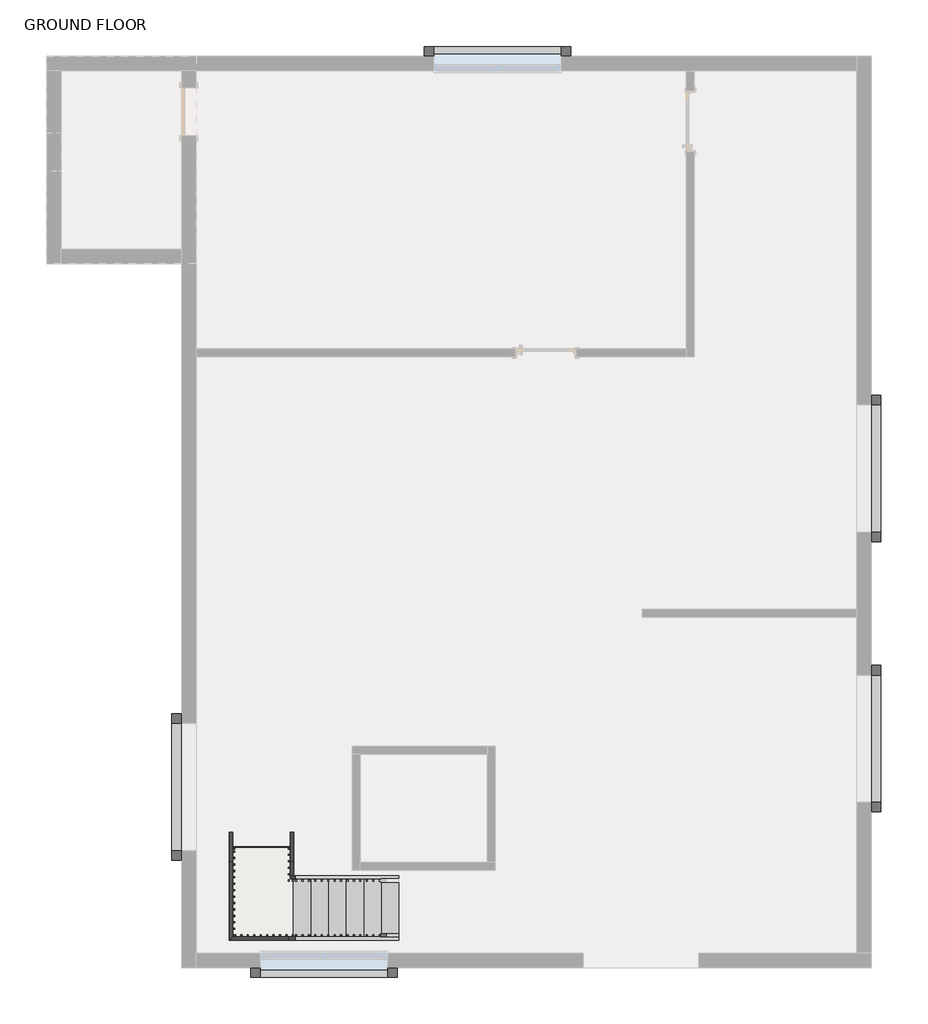
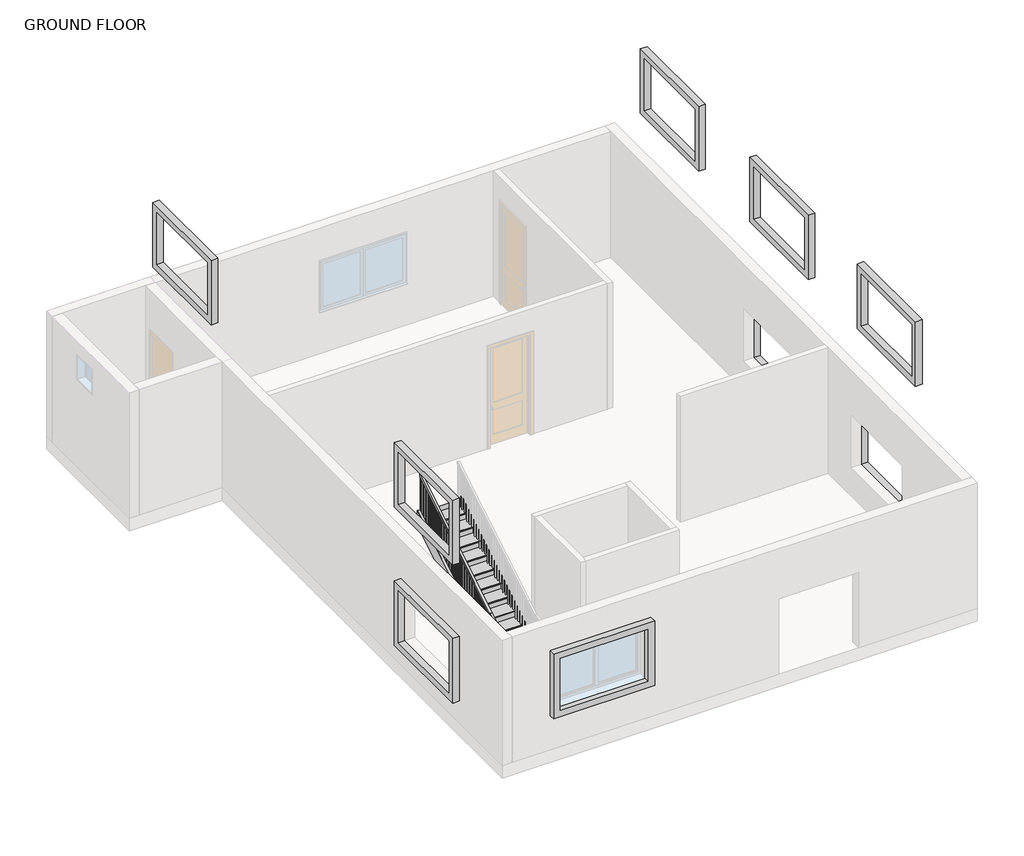
# One storey, part 2 of 2: 7 members, 4 proxies, 2 stair flights, 1 railing, 1 slab.
"""IFC4 building model written with IfcOpenShell, lengths in millimetres."""

from ifc_helpers import new_model, si_unit, frame, origin, place, context, project, spatial, polyline, outline, extrude, faceted_brep, transform, mapped, element, save
from components import generic_models_3_generic_models_3_62885dc4, generic_models_4_generic_models_4_3a3d2180, generic_models_7_generic_models_7_0c2edacf, generic_models_8_generic_models_8_56cf2c1e, non_monolithic_landing_e724ba9d, stair_flight_0804820e, stair_flight_c801c68a

model = new_model("IFC4")

# Units and contexts
model_context = context("Model", 3, world=origin())
ifc_project = project(units=[si_unit("LENGTHUNIT", "METRE", prefix="MILLI")], contexts=[model_context])

# Site, building, storey
site = spatial("IfcSite", under=ifc_project)
building = spatial("IfcBuilding", under=site)
storey = spatial("IfcBuildingStorey", under=building, Name="GROUND FLOOR", Elevation=304.8)

# Proxies
placement = place(None, origin())
generic_models_3_generic_models_3_shape = generic_models_3_generic_models_3_62885dc4(model_context)
element("IfcBuildingElementProxy", 1, Name="Generic Models 3 : Generic Models 3", ObjectType="Generic Models 3 : Generic Models 3", at=placement, inside=storey, context=model_context, shape_type="MappedRepresentation", body=[
    mapped(generic_models_3_generic_models_3_shape, transform((0.0, 0.0, 0.0), x_axis=(1.0, 0.0, 0.0), y_axis=(0.0, 1.0, 0.0), z_axis=(0.0, 0.0, 1.0))),
])
generic_models_4_generic_models_4_shape = generic_models_4_generic_models_4_3a3d2180(model_context)
element("IfcBuildingElementProxy", 2, Name="Generic Models 4 : Generic Models 4", ObjectType="Generic Models 4 : Generic Models 4", at=placement, inside=storey, context=model_context, shape_type="MappedRepresentation", body=[
    mapped(generic_models_4_generic_models_4_shape, transform((0.0, 0.0, 0.0), x_axis=(1.0, 0.0, 0.0), y_axis=(0.0, 1.0, 0.0), z_axis=(0.0, 0.0, 1.0))),
])
generic_models_7_generic_models_7_shape = generic_models_7_generic_models_7_0c2edacf(model_context)
element("IfcBuildingElementProxy", 3, Name="Generic Models 7 : Generic Models 7", ObjectType="Generic Models 7 : Generic Models 7", at=placement, inside=storey, context=model_context, shape_type="MappedRepresentation", body=[
    mapped(generic_models_7_generic_models_7_shape, transform((0.0, 0.0, 0.0), x_axis=(1.0, 0.0, 0.0), y_axis=(0.0, 1.0, 0.0), z_axis=(0.0, 0.0, 1.0))),
])
generic_models_8_generic_models_8_shape = generic_models_8_generic_models_8_56cf2c1e(model_context)
element("IfcBuildingElementProxy", 4, Name="Generic Models 8 : Generic Models 8", ObjectType="Generic Models 8 : Generic Models 8", at=placement, inside=storey, context=model_context, shape_type="MappedRepresentation", body=[
    mapped(generic_models_8_generic_models_8_shape, transform((0.0, 0.0, 0.0), x_axis=(1.0, 0.0, 0.0), y_axis=(0.0, 1.0, 0.0), z_axis=(0.0, 0.0, 1.0))),
])

# Members
element("IfcMember", 5, ObjectType="Stringer - 2\" Width", at=placement, inside=storey, context=model_context, shape_type="SweptSolid", body=[
    extrude(outline(polyline([(304.8, -3322.4601025), (516.914512, -3322.4601025), (1566.3333333, -5054.0011578), (1261.5333333, -5139.1556143), (304.8, -3560.5456143), (304.8, -3322.4601025)])), frame((0.0, -3834.257314, 0.0), z_axis=(0.0, 1.0, 0.0), x_axis=(0.0, 0.0, 1.0)), (0.0, 0.0, 1.0), 50.8),
])
element("IfcMember", 6, ObjectType="Stringer - 2\" Width", at=placement, inside=storey, context=model_context, shape_type="SweptSolid", body=[
    extrude(outline(polyline([(304.8, -3322.4601025), (516.914512, -3322.4601025), (1556.1357187, -5037.1750936), (1199.7269571, -5037.1750936), (304.8, -3560.5456143), (304.8, -3322.4601025)])), frame((0.0, -2869.057314, 0.0), z_axis=(0.0, 1.0, 0.0), x_axis=(0.0, 0.0, 1.0)), (0.0, 0.0, 1.0), 50.8),
])
element("IfcMember", 7, ObjectType="Stringer - 2\" Width", at=placement, inside=storey, context=model_context, shape_type="SweptSolid", body=[
    extrude(outline(polyline([(-2530.2317367, 1261.5333333), (-2615.3861932, 1566.3333333), (402.8727516, 3395.5811786), (402.8727516, 3039.1724171), (-2530.2317367, 1261.5333333)])), frame((-6002.3750936, 0.0, 0.0), z_axis=(1.0, 0.0, 0.0), x_axis=(0.0, 1.0, 0.0)), (0.0, 0.0, 1.0), 50.8),
])
element("IfcMember", 8, ObjectType="Stringer - 2\" Width", at=placement, inside=storey, context=model_context, shape_type="SweptSolid", body=[
    extrude(outline(polyline([(-2530.2317367, 1261.5333333), (-2615.3861932, 1566.3333333), (402.8727516, 3395.5811786), (402.8727516, 3039.1724171), (-2530.2317367, 1261.5333333)])), frame((-5037.1750936, 0.0, 0.0), z_axis=(1.0, 0.0, 0.0), x_axis=(0.0, 1.0, 0.0)), (0.0, 0.0, 1.0), 50.8),
])
element("IfcMember", 9, ObjectType="Stringer - 2\" Width", at=placement, inside=storey, context=model_context, shape_type="Brep", body=[
    faceted_brep([(-5951.5750936, -2615.3861932, 1566.3333333), (-6002.3750936, -2615.3861932, 1566.3333333), (-6002.3750936, -3834.257314, 1566.3333333), (-5951.5750936, -3783.457314, 1566.3333333), (-5951.5750936, -2530.2317367, 1261.5333333), (-5951.5750936, -3783.457314, 1261.5333333), (-6002.3750936, -2530.2317367, 1261.5333333), (-6002.3750936, -3834.257314, 1261.5333333)], [[[0, 1, 2, 3]], [[4, 0, 3, 5]], [[6, 4, 5, 7]], [[1, 6, 7, 2]], [[1, 0, 4, 6]], [[2, 7, 5, 3]]]),
])
element("IfcMember", 10, ObjectType="Stringer - 2\" Width", at=placement, inside=storey, context=model_context, shape_type="Brep", body=[
    faceted_brep([(-5951.5750936, -3783.457314, 1566.3333333), (-6002.3750936, -3834.257314, 1566.3333333), (-5054.0011578, -3834.257314, 1566.3333333), (-5054.0011578, -3783.457314, 1566.3333333), (-5951.5750936, -3783.457314, 1261.5333333), (-5139.1556143, -3783.457314, 1261.5333333), (-6002.3750936, -3834.257314, 1261.5333333), (-5139.1556143, -3834.257314, 1261.5333333)], [[[0, 1, 2, 3]], [[4, 0, 3, 5]], [[6, 4, 5, 7]], [[1, 6, 7, 2]], [[1, 0, 4, 6]], [[2, 7, 5, 3]]]),
])
element("IfcMember", 11, ObjectType="Stringer - 2\" Width", at=placement, inside=storey, context=model_context, shape_type="SweptSolid", body=[
    extrude(outline(polyline([(-2818.257314, 1261.5333333), (-2818.257314, 1566.3333333), (-2615.3861932, 1566.3333333), (-2530.2317367, 1261.5333333), (-2818.257314, 1261.5333333)])), frame((-5037.1750936, 0.0, 0.0), z_axis=(1.0, 0.0, 0.0), x_axis=(0.0, 1.0, 0.0)), (0.0, 0.0, 1.0), 50.8),
])

# Railing
element("IfcRailing", 12, ObjectType="Handrail - Rectangular", at=placement, inside=storey, context=model_context, shape_type="SolidModel", body=[
    faceted_brep([(-3322.4601025, -3783.457314, 1388.5333333), (-3322.4601025, -3783.457314, 1329.1318731), (-3322.4601025, -3732.657314, 1329.1318731), (-3322.4601025, -3732.657314, 1388.5333333), (-4998.8601025, -3783.457314, 2404.5333333), (-5013.0525119, -3783.457314, 2353.7333333), (-5013.0525119, -3732.657314, 2353.7333333), (-4998.8601025, -3732.657314, 2404.5333333), (-5951.5750936, -3783.457314, 2404.5333333), (-5951.5750936, -3783.457314, 2353.7333333), (-5900.7750936, -3732.657314, 2353.7333333), (-5900.7750936, -3732.657314, 2404.5333333), (-5951.5750936, -2670.5272484, 2404.5333333), (-5951.5750936, -2656.334839, 2353.7333333), (-5900.7750936, -2656.334839, 2353.7333333), (-5900.7750936, -2670.5272484, 2404.5333333), (-5951.5750936, -2391.1272484, 2573.8666667), (-5951.5750936, -2364.7975213, 2530.4226168), (-5900.7750936, -2364.7975213, 2530.4226168), (-5900.7750936, -2391.1272484, 2573.8666667), (-5951.5750936, 402.8727516, 4267.2), (-5900.7750936, 402.8727516, 4267.2), (-5900.7750936, 402.8727516, 4207.7985397), (-5951.5750936, 402.8727516, 4207.7985397)], [[[0, 1, 2, 3]], [[1, 0, 4, 5]], [[2, 1, 5, 6]], [[3, 2, 6, 7]], [[0, 3, 7, 4]], [[5, 4, 8, 9]], [[6, 5, 9, 10]], [[7, 6, 10, 11]], [[4, 7, 11, 8]], [[9, 8, 12, 13]], [[10, 9, 13, 14]], [[11, 10, 14, 15]], [[8, 11, 15, 12]], [[13, 12, 16, 17]], [[14, 13, 17, 18]], [[15, 14, 18, 19]], [[12, 15, 19, 16]], [[20, 21, 22, 23]], [[17, 16, 20, 23]], [[18, 17, 23, 22]], [[19, 18, 22, 21]], [[16, 19, 21, 20]]]),
    extrude(outline(polyline([(361.5977516, 4182.7833882), (361.5977516, 3183.4666667), (342.5477516, 3183.4666667), (342.5477516, 4171.2379337), (361.5977516, 4182.7833882)])), frame((-5935.7000936, 0.0, 0.0), z_axis=(1.0, 0.0, 0.0), x_axis=(0.0, 1.0, 0.0)), (0.0, 0.0, 1.0), 19.05),
    extrude(outline(polyline([(259.9977516, 4121.2076307), (259.9977516, 3183.4666667), (240.9477516, 3183.4666667), (240.9477516, 4109.6621761), (259.9977516, 4121.2076307)])), frame((-5935.7000936, 0.0, 0.0), z_axis=(1.0, 0.0, 0.0), x_axis=(0.0, 1.0, 0.0)), (0.0, 0.0, 1.0), 19.05),
    extrude(outline(polyline([(158.3977516, 4059.6318731), (158.3977516, 3183.4666667), (139.3477516, 3183.4666667), (139.3477516, 4048.0864185), (158.3977516, 4059.6318731)])), frame((-5935.7000936, 0.0, 0.0), z_axis=(1.0, 0.0, 0.0), x_axis=(0.0, 1.0, 0.0)), (0.0, 0.0, 1.0), 19.05),
    extrude(outline(polyline([(56.7977516, 3998.0561155), (56.7977516, 3014.1333333), (37.7477516, 3014.1333333), (37.7477516, 3986.510661), (56.7977516, 3998.0561155)])), frame((-5935.7000936, 0.0, 0.0), z_axis=(1.0, 0.0, 0.0), x_axis=(0.0, 1.0, 0.0)), (0.0, 0.0, 1.0), 19.05),
    extrude(outline(polyline([(-44.8022484, 3936.4803579), (-44.8022484, 3014.1333333), (-63.8522484, 3014.1333333), (-63.8522484, 3924.9349034), (-44.8022484, 3936.4803579)])), frame((-5935.7000936, 0.0, 0.0), z_axis=(1.0, 0.0, 0.0), x_axis=(0.0, 1.0, 0.0)), (0.0, 0.0, 1.0), 19.05),
    extrude(outline(polyline([(-146.4022484, 3874.9046004), (-146.4022484, 3014.1333333), (-165.4522484, 3014.1333333), (-165.4522484, 3863.3591458), (-146.4022484, 3874.9046004)])), frame((-5935.7000936, 0.0, 0.0), z_axis=(1.0, 0.0, 0.0), x_axis=(0.0, 1.0, 0.0)), (0.0, 0.0, 1.0), 19.05),
    extrude(outline(polyline([(-248.0022484, 3813.3288428), (-248.0022484, 2844.8), (-267.0522484, 2844.8), (-267.0522484, 3801.7833882), (-248.0022484, 3813.3288428)])), frame((-5935.7000936, 0.0, 0.0), z_axis=(1.0, 0.0, 0.0), x_axis=(0.0, 1.0, 0.0)), (0.0, 0.0, 1.0), 19.05),
    extrude(outline(polyline([(-349.6022484, 3751.7530852), (-349.6022484, 2844.8), (-368.6522484, 2844.8), (-368.6522484, 3740.2076307), (-349.6022484, 3751.7530852)])), frame((-5935.7000936, 0.0, 0.0), z_axis=(1.0, 0.0, 0.0), x_axis=(0.0, 1.0, 0.0)), (0.0, 0.0, 1.0), 19.05),
    extrude(outline(polyline([(-451.2022484, 3690.1773276), (-451.2022484, 2675.4666667), (-470.2522484, 2675.4666667), (-470.2522484, 3678.6318731), (-451.2022484, 3690.1773276)])), frame((-5935.7000936, 0.0, 0.0), z_axis=(1.0, 0.0, 0.0), x_axis=(0.0, 1.0, 0.0)), (0.0, 0.0, 1.0), 19.05),
    extrude(outline(polyline([(-552.8022484, 3628.60157), (-552.8022484, 2675.4666667), (-571.8522484, 2675.4666667), (-571.8522484, 3617.0561155), (-552.8022484, 3628.60157)])), frame((-5935.7000936, 0.0, 0.0), z_axis=(1.0, 0.0, 0.0), x_axis=(0.0, 1.0, 0.0)), (0.0, 0.0, 1.0), 19.05),
    extrude(outline(polyline([(-654.4022484, 3567.0258125), (-654.4022484, 2675.4666667), (-673.4522484, 2675.4666667), (-673.4522484, 3555.4803579), (-654.4022484, 3567.0258125)])), frame((-5935.7000936, 0.0, 0.0), z_axis=(1.0, 0.0, 0.0), x_axis=(0.0, 1.0, 0.0)), (0.0, 0.0, 1.0), 19.05),
    extrude(outline(polyline([(-756.0022484, 3505.4500549), (-756.0022484, 2506.1333333), (-775.0522484, 2506.1333333), (-775.0522484, 3493.9046004), (-756.0022484, 3505.4500549)])), frame((-5935.7000936, 0.0, 0.0), z_axis=(1.0, 0.0, 0.0), x_axis=(0.0, 1.0, 0.0)), (0.0, 0.0, 1.0), 19.05),
    extrude(outline(polyline([(-857.6022484, 3443.8742973), (-857.6022484, 2506.1333333), (-876.6522484, 2506.1333333), (-876.6522484, 3432.3288428), (-857.6022484, 3443.8742973)])), frame((-5935.7000936, 0.0, 0.0), z_axis=(1.0, 0.0, 0.0), x_axis=(0.0, 1.0, 0.0)), (0.0, 0.0, 1.0), 19.05),
    extrude(outline(polyline([(-959.2022484, 3382.2985397), (-959.2022484, 2506.1333333), (-978.2522484, 2506.1333333), (-978.2522484, 3370.7530852), (-959.2022484, 3382.2985397)])), frame((-5935.7000936, 0.0, 0.0), z_axis=(1.0, 0.0, 0.0), x_axis=(0.0, 1.0, 0.0)), (0.0, 0.0, 1.0), 19.05),
    extrude(outline(polyline([(-1060.8022484, 3320.7227822), (-1060.8022484, 2336.8), (-1079.8522484, 2336.8), (-1079.8522484, 3309.1773276), (-1060.8022484, 3320.7227822)])), frame((-5935.7000936, 0.0, 0.0), z_axis=(1.0, 0.0, 0.0), x_axis=(0.0, 1.0, 0.0)), (0.0, 0.0, 1.0), 19.05),
    extrude(outline(polyline([(-1162.4022484, 3259.1470246), (-1162.4022484, 2336.8), (-1181.4522484, 2336.8), (-1181.4522484, 3247.60157), (-1162.4022484, 3259.1470246)])), frame((-5935.7000936, 0.0, 0.0), z_axis=(1.0, 0.0, 0.0), x_axis=(0.0, 1.0, 0.0)), (0.0, 0.0, 1.0), 19.05),
    extrude(outline(polyline([(-1264.0022484, 3197.571267), (-1264.0022484, 2336.8), (-1283.0522484, 2336.8), (-1283.0522484, 3186.0258125), (-1264.0022484, 3197.571267)])), frame((-5935.7000936, 0.0, 0.0), z_axis=(1.0, 0.0, 0.0), x_axis=(0.0, 1.0, 0.0)), (0.0, 0.0, 1.0), 19.05),
    extrude(outline(polyline([(-1365.6022484, 3135.9955094), (-1365.6022484, 2167.4666667), (-1384.6522484, 2167.4666667), (-1384.6522484, 3124.4500549), (-1365.6022484, 3135.9955094)])), frame((-5935.7000936, 0.0, 0.0), z_axis=(1.0, 0.0, 0.0), x_axis=(0.0, 1.0, 0.0)), (0.0, 0.0, 1.0), 19.05),
    extrude(outline(polyline([(-1467.2022484, 3074.4197519), (-1467.2022484, 2167.4666667), (-1486.2522484, 2167.4666667), (-1486.2522484, 3062.8742973), (-1467.2022484, 3074.4197519)])), frame((-5935.7000936, 0.0, 0.0), z_axis=(1.0, 0.0, 0.0), x_axis=(0.0, 1.0, 0.0)), (0.0, 0.0, 1.0), 19.05),
    extrude(outline(polyline([(-1568.8022484, 3012.8439943), (-1568.8022484, 1998.1333333), (-1587.8522484, 1998.1333333), (-1587.8522484, 3001.2985397), (-1568.8022484, 3012.8439943)])), frame((-5935.7000936, 0.0, 0.0), z_axis=(1.0, 0.0, 0.0), x_axis=(0.0, 1.0, 0.0)), (0.0, 0.0, 1.0), 19.05),
    extrude(outline(polyline([(-1670.4022484, 2951.2682367), (-1670.4022484, 1998.1333333), (-1689.4522484, 1998.1333333), (-1689.4522484, 2939.7227822), (-1670.4022484, 2951.2682367)])), frame((-5935.7000936, 0.0, 0.0), z_axis=(1.0, 0.0, 0.0), x_axis=(0.0, 1.0, 0.0)), (0.0, 0.0, 1.0), 19.05),
    extrude(outline(polyline([(-1772.0022484, 2889.6924791), (-1772.0022484, 1998.1333333), (-1791.0522484, 1998.1333333), (-1791.0522484, 2878.1470246), (-1772.0022484, 2889.6924791)])), frame((-5935.7000936, 0.0, 0.0), z_axis=(1.0, 0.0, 0.0), x_axis=(0.0, 1.0, 0.0)), (0.0, 0.0, 1.0), 19.05),
    extrude(outline(polyline([(-1873.6022484, 2828.1167216), (-1873.6022484, 1828.8), (-1892.6522484, 1828.8), (-1892.6522484, 2816.571267), (-1873.6022484, 2828.1167216)])), frame((-5935.7000936, 0.0, 0.0), z_axis=(1.0, 0.0, 0.0), x_axis=(0.0, 1.0, 0.0)), (0.0, 0.0, 1.0), 19.05),
    extrude(outline(polyline([(-1975.2022484, 2766.540964), (-1975.2022484, 1828.8), (-1994.2522484, 1828.8), (-1994.2522484, 2754.9955094), (-1975.2022484, 2766.540964)])), frame((-5935.7000936, 0.0, 0.0), z_axis=(1.0, 0.0, 0.0), x_axis=(0.0, 1.0, 0.0)), (0.0, 0.0, 1.0), 19.05),
    extrude(outline(polyline([(-2076.8022484, 2704.9652064), (-2076.8022484, 1828.8), (-2095.8522484, 1828.8), (-2095.8522484, 2693.4197519), (-2076.8022484, 2704.9652064)])), frame((-5935.7000936, 0.0, 0.0), z_axis=(1.0, 0.0, 0.0), x_axis=(0.0, 1.0, 0.0)), (0.0, 0.0, 1.0), 19.05),
    extrude(outline(polyline([(-2178.4022484, 2643.3894488), (-2178.4022484, 1659.4666667), (-2197.4522484, 1659.4666667), (-2197.4522484, 2631.8439943), (-2178.4022484, 2643.3894488)])), frame((-5935.7000936, 0.0, 0.0), z_axis=(1.0, 0.0, 0.0), x_axis=(0.0, 1.0, 0.0)), (0.0, 0.0, 1.0), 19.05),
    extrude(outline(polyline([(-2280.0022484, 2581.8136913), (-2280.0022484, 1659.4666667), (-2299.0522484, 1659.4666667), (-2299.0522484, 2570.2682367), (-2280.0022484, 2581.8136913)])), frame((-5935.7000936, 0.0, 0.0), z_axis=(1.0, 0.0, 0.0), x_axis=(0.0, 1.0, 0.0)), (0.0, 0.0, 1.0), 19.05),
    extrude(outline(polyline([(-2427.732314, 2492.2803182), (-2427.732314, 1490.1333333), (-2446.782314, 1490.1333333), (-2446.782314, 2480.7348636), (-2427.732314, 2492.2803182)])), frame((-5935.7000936, 0.0, 0.0), z_axis=(1.0, 0.0, 0.0), x_axis=(0.0, 1.0, 0.0)), (0.0, 0.0, 1.0), 19.05),
    extrude(outline(polyline([(-2529.332314, 2430.7045606), (-2529.332314, 1490.1333333), (-2548.382314, 1490.1333333), (-2548.382314, 2419.1591061), (-2529.332314, 2430.7045606)])), frame((-5935.7000936, 0.0, 0.0), z_axis=(1.0, 0.0, 0.0), x_axis=(0.0, 1.0, 0.0)), (0.0, 0.0, 1.0), 19.05),
    extrude(outline(polyline([(-2630.932314, 2369.128803), (-2630.932314, 1490.1333333), (-2649.982314, 1490.1333333), (-2649.982314, 2357.5833485), (-2630.932314, 2369.128803)])), frame((-5935.7000936, 0.0, 0.0), z_axis=(1.0, 0.0, 0.0), x_axis=(0.0, 1.0, 0.0)), (0.0, 0.0, 1.0), 19.05),
    extrude(outline(polyline([(-5935.7000936, -2751.582314), (-5935.7000936, -2732.532314), (-5916.6500936, -2732.532314), (-5916.6500936, -2751.582314), (-5935.7000936, -2751.582314)])), frame((0.0, 0.0, 1490.1333333), z_axis=(0.0, 0.0, 1.0), x_axis=(1.0, 0.0, 0.0)), (0.0, 0.0, 1.0), 863.6),
    extrude(outline(polyline([(-5935.7000936, -2853.182314), (-5935.7000936, -2834.132314), (-5916.6500936, -2834.132314), (-5916.6500936, -2853.182314), (-5935.7000936, -2853.182314)])), frame((0.0, 0.0, 1490.1333333), z_axis=(0.0, 0.0, 1.0), x_axis=(1.0, 0.0, 0.0)), (0.0, 0.0, 1.0), 863.6),
    extrude(outline(polyline([(-5935.7000936, -2954.782314), (-5935.7000936, -2935.732314), (-5916.6500936, -2935.732314), (-5916.6500936, -2954.782314), (-5935.7000936, -2954.782314)])), frame((0.0, 0.0, 1490.1333333), z_axis=(0.0, 0.0, 1.0), x_axis=(1.0, 0.0, 0.0)), (0.0, 0.0, 1.0), 863.6),
    extrude(outline(polyline([(-5935.7000936, -3056.382314), (-5935.7000936, -3037.332314), (-5916.6500936, -3037.332314), (-5916.6500936, -3056.382314), (-5935.7000936, -3056.382314)])), frame((0.0, 0.0, 1490.1333333), z_axis=(0.0, 0.0, 1.0), x_axis=(1.0, 0.0, 0.0)), (0.0, 0.0, 1.0), 863.6),
    extrude(outline(polyline([(-5935.7000936, -3157.982314), (-5935.7000936, -3138.932314), (-5916.6500936, -3138.932314), (-5916.6500936, -3157.982314), (-5935.7000936, -3157.982314)])), frame((0.0, 0.0, 1490.1333333), z_axis=(0.0, 0.0, 1.0), x_axis=(1.0, 0.0, 0.0)), (0.0, 0.0, 1.0), 863.6),
    extrude(outline(polyline([(-5935.7000936, -3259.582314), (-5935.7000936, -3240.532314), (-5916.6500936, -3240.532314), (-5916.6500936, -3259.582314), (-5935.7000936, -3259.582314)])), frame((0.0, 0.0, 1490.1333333), z_axis=(0.0, 0.0, 1.0), x_axis=(1.0, 0.0, 0.0)), (0.0, 0.0, 1.0), 863.6),
    extrude(outline(polyline([(-5935.7000936, -3361.182314), (-5935.7000936, -3342.132314), (-5916.6500936, -3342.132314), (-5916.6500936, -3361.182314), (-5935.7000936, -3361.182314)])), frame((0.0, 0.0, 1490.1333333), z_axis=(0.0, 0.0, 1.0), x_axis=(1.0, 0.0, 0.0)), (0.0, 0.0, 1.0), 863.6),
    extrude(outline(polyline([(-5935.7000936, -3462.782314), (-5935.7000936, -3443.732314), (-5916.6500936, -3443.732314), (-5916.6500936, -3462.782314), (-5935.7000936, -3462.782314)])), frame((0.0, 0.0, 1490.1333333), z_axis=(0.0, 0.0, 1.0), x_axis=(1.0, 0.0, 0.0)), (0.0, 0.0, 1.0), 863.6),
    extrude(outline(polyline([(-5935.7000936, -3564.382314), (-5935.7000936, -3545.332314), (-5916.6500936, -3545.332314), (-5916.6500936, -3564.382314), (-5935.7000936, -3564.382314)])), frame((0.0, 0.0, 1490.1333333), z_axis=(0.0, 0.0, 1.0), x_axis=(1.0, 0.0, 0.0)), (0.0, 0.0, 1.0), 863.6),
    extrude(outline(polyline([(-5935.7000936, -3665.982314), (-5935.7000936, -3646.932314), (-5916.6500936, -3646.932314), (-5916.6500936, -3665.982314), (-5935.7000936, -3665.982314)])), frame((0.0, 0.0, 1490.1333333), z_axis=(0.0, 0.0, 1.0), x_axis=(1.0, 0.0, 0.0)), (0.0, 0.0, 1.0), 863.6),
    extrude(outline(polyline([(-5903.7351025, -3767.582314), (-5922.7851025, -3767.582314), (-5922.7851025, -3748.532314), (-5903.7351025, -3748.532314), (-5903.7351025, -3767.582314)])), frame((0.0, 0.0, 1490.1333333), z_axis=(0.0, 0.0, 1.0), x_axis=(1.0, 0.0, 0.0)), (0.0, 0.0, 1.0), 863.6),
    extrude(outline(polyline([(-5802.1351025, -3767.582314), (-5821.1851025, -3767.582314), (-5821.1851025, -3748.532314), (-5802.1351025, -3748.532314), (-5802.1351025, -3767.582314)])), frame((0.0, 0.0, 1490.1333333), z_axis=(0.0, 0.0, 1.0), x_axis=(1.0, 0.0, 0.0)), (0.0, 0.0, 1.0), 863.6),
    extrude(outline(polyline([(-5700.5351025, -3767.582314), (-5719.5851025, -3767.582314), (-5719.5851025, -3748.532314), (-5700.5351025, -3748.532314), (-5700.5351025, -3767.582314)])), frame((0.0, 0.0, 1490.1333333), z_axis=(0.0, 0.0, 1.0), x_axis=(1.0, 0.0, 0.0)), (0.0, 0.0, 1.0), 863.6),
    extrude(outline(polyline([(-5598.9351025, -3767.582314), (-5617.9851025, -3767.582314), (-5617.9851025, -3748.532314), (-5598.9351025, -3748.532314), (-5598.9351025, -3767.582314)])), frame((0.0, 0.0, 1490.1333333), z_axis=(0.0, 0.0, 1.0), x_axis=(1.0, 0.0, 0.0)), (0.0, 0.0, 1.0), 863.6),
    extrude(outline(polyline([(-5497.3351025, -3767.582314), (-5516.3851025, -3767.582314), (-5516.3851025, -3748.532314), (-5497.3351025, -3748.532314), (-5497.3351025, -3767.582314)])), frame((0.0, 0.0, 1490.1333333), z_axis=(0.0, 0.0, 1.0), x_axis=(1.0, 0.0, 0.0)), (0.0, 0.0, 1.0), 863.6),
    extrude(outline(polyline([(-5395.7351025, -3767.582314), (-5414.7851025, -3767.582314), (-5414.7851025, -3748.532314), (-5395.7351025, -3748.532314), (-5395.7351025, -3767.582314)])), frame((0.0, 0.0, 1490.1333333), z_axis=(0.0, 0.0, 1.0), x_axis=(1.0, 0.0, 0.0)), (0.0, 0.0, 1.0), 863.6),
    extrude(outline(polyline([(-5294.1351025, -3767.582314), (-5313.1851025, -3767.582314), (-5313.1851025, -3748.532314), (-5294.1351025, -3748.532314), (-5294.1351025, -3767.582314)])), frame((0.0, 0.0, 1490.1333333), z_axis=(0.0, 0.0, 1.0), x_axis=(1.0, 0.0, 0.0)), (0.0, 0.0, 1.0), 863.6),
    extrude(outline(polyline([(-5192.5351025, -3767.582314), (-5211.5851025, -3767.582314), (-5211.5851025, -3748.532314), (-5192.5351025, -3748.532314), (-5192.5351025, -3767.582314)])), frame((0.0, 0.0, 1490.1333333), z_axis=(0.0, 0.0, 1.0), x_axis=(1.0, 0.0, 0.0)), (0.0, 0.0, 1.0), 863.6),
    extrude(outline(polyline([(-5090.9351025, -3767.582314), (-5109.9851025, -3767.582314), (-5109.9851025, -3748.532314), (-5090.9351025, -3748.532314), (-5090.9351025, -3767.582314)])), frame((0.0, 0.0, 1490.1333333), z_axis=(0.0, 0.0, 1.0), x_axis=(1.0, 0.0, 0.0)), (0.0, 0.0, 1.0), 863.6),
    extrude(outline(polyline([(2320.1167216, -4957.5851025), (1320.8, -4957.5851025), (1320.8, -4938.5351025), (2308.571267, -4938.5351025), (2320.1167216, -4957.5851025)])), frame((0.0, -3767.582314, 0.0), z_axis=(0.0, 1.0, 0.0), x_axis=(0.0, 0.0, 1.0)), (0.0, 0.0, 1.0), 19.05),
    extrude(outline(polyline([(2258.540964, -4855.9851025), (1320.8, -4855.9851025), (1320.8, -4836.9351025), (2246.9955094, -4836.9351025), (2258.540964, -4855.9851025)])), frame((0.0, -3767.582314, 0.0), z_axis=(0.0, 1.0, 0.0), x_axis=(0.0, 0.0, 1.0)), (0.0, 0.0, 1.0), 19.05),
    extrude(outline(polyline([(2196.9652064, -4754.3851025), (1320.8, -4754.3851025), (1320.8, -4735.3351025), (2185.4197519, -4735.3351025), (2196.9652064, -4754.3851025)])), frame((0.0, -3767.582314, 0.0), z_axis=(0.0, 1.0, 0.0), x_axis=(0.0, 0.0, 1.0)), (0.0, 0.0, 1.0), 19.05),
    extrude(outline(polyline([(2135.3894488, -4652.7851025), (1151.4666667, -4652.7851025), (1151.4666667, -4633.7351025), (2123.8439943, -4633.7351025), (2135.3894488, -4652.7851025)])), frame((0.0, -3767.582314, 0.0), z_axis=(0.0, 1.0, 0.0), x_axis=(0.0, 0.0, 1.0)), (0.0, 0.0, 1.0), 19.05),
    extrude(outline(polyline([(2073.8136913, -4551.1851025), (1151.4666667, -4551.1851025), (1151.4666667, -4532.1351025), (2062.2682367, -4532.1351025), (2073.8136913, -4551.1851025)])), frame((0.0, -3767.582314, 0.0), z_axis=(0.0, 1.0, 0.0), x_axis=(0.0, 0.0, 1.0)), (0.0, 0.0, 1.0), 19.05),
    extrude(outline(polyline([(2012.2379337, -4449.5851025), (1151.4666667, -4449.5851025), (1151.4666667, -4430.5351025), (2000.6924791, -4430.5351025), (2012.2379337, -4449.5851025)])), frame((0.0, -3767.582314, 0.0), z_axis=(0.0, 1.0, 0.0), x_axis=(0.0, 0.0, 1.0)), (0.0, 0.0, 1.0), 19.05),
    extrude(outline(polyline([(1950.6621761, -4347.9851025), (982.1333333, -4347.9851025), (982.1333333, -4328.9351025), (1939.1167216, -4328.9351025), (1950.6621761, -4347.9851025)])), frame((0.0, -3767.582314, 0.0), z_axis=(0.0, 1.0, 0.0), x_axis=(0.0, 0.0, 1.0)), (0.0, 0.0, 1.0), 19.05),
    extrude(outline(polyline([(1889.0864185, -4246.3851025), (982.1333333, -4246.3851025), (982.1333333, -4227.3351025), (1877.540964, -4227.3351025), (1889.0864185, -4246.3851025)])), frame((0.0, -3767.582314, 0.0), z_axis=(0.0, 1.0, 0.0), x_axis=(0.0, 0.0, 1.0)), (0.0, 0.0, 1.0), 19.05),
    extrude(outline(polyline([(1827.510661, -4144.7851025), (812.8, -4144.7851025), (812.8, -4125.7351025), (1815.9652064, -4125.7351025), (1827.510661, -4144.7851025)])), frame((0.0, -3767.582314, 0.0), z_axis=(0.0, 1.0, 0.0), x_axis=(0.0, 0.0, 1.0)), (0.0, 0.0, 1.0), 19.05),
    extrude(outline(polyline([(1765.9349034, -4043.1851025), (812.8, -4043.1851025), (812.8, -4024.1351025), (1754.3894488, -4024.1351025), (1765.9349034, -4043.1851025)])), frame((0.0, -3767.582314, 0.0), z_axis=(0.0, 1.0, 0.0), x_axis=(0.0, 0.0, 1.0)), (0.0, 0.0, 1.0), 19.05),
    extrude(outline(polyline([(1704.3591458, -3941.5851025), (812.8, -3941.5851025), (812.8, -3922.5351025), (1692.8136913, -3922.5351025), (1704.3591458, -3941.5851025)])), frame((0.0, -3767.582314, 0.0), z_axis=(0.0, 1.0, 0.0), x_axis=(0.0, 0.0, 1.0)), (0.0, 0.0, 1.0), 19.05),
    extrude(outline(polyline([(1642.7833882, -3839.9851025), (643.4666667, -3839.9851025), (643.4666667, -3820.9351025), (1631.2379337, -3820.9351025), (1642.7833882, -3839.9851025)])), frame((0.0, -3767.582314, 0.0), z_axis=(0.0, 1.0, 0.0), x_axis=(0.0, 0.0, 1.0)), (0.0, 0.0, 1.0), 19.05),
    extrude(outline(polyline([(1581.2076307, -3738.3851025), (643.4666667, -3738.3851025), (643.4666667, -3719.3351025), (1569.6621761, -3719.3351025), (1581.2076307, -3738.3851025)])), frame((0.0, -3767.582314, 0.0), z_axis=(0.0, 1.0, 0.0), x_axis=(0.0, 0.0, 1.0)), (0.0, 0.0, 1.0), 19.05),
    extrude(outline(polyline([(1519.6318731, -3636.7851025), (643.4666667, -3636.7851025), (643.4666667, -3617.7351025), (1508.0864185, -3617.7351025), (1519.6318731, -3636.7851025)])), frame((0.0, -3767.582314, 0.0), z_axis=(0.0, 1.0, 0.0), x_axis=(0.0, 0.0, 1.0)), (0.0, 0.0, 1.0), 19.05),
    extrude(outline(polyline([(1458.0561155, -3535.1851025), (474.1333333, -3535.1851025), (474.1333333, -3516.1351025), (1446.510661, -3516.1351025), (1458.0561155, -3535.1851025)])), frame((0.0, -3767.582314, 0.0), z_axis=(0.0, 1.0, 0.0), x_axis=(0.0, 0.0, 1.0)), (0.0, 0.0, 1.0), 19.05),
    extrude(outline(polyline([(1396.4803579, -3433.5851025), (474.1333333, -3433.5851025), (474.1333333, -3414.5351025), (1384.9349034, -3414.5351025), (1396.4803579, -3433.5851025)])), frame((0.0, -3767.582314, 0.0), z_axis=(0.0, 1.0, 0.0), x_axis=(0.0, 0.0, 1.0)), (0.0, 0.0, 1.0), 19.05),
    extrude(outline(polyline([(-2381.6022484, 2520.2379337), (-2381.6022484, 1490.1333333), (-2400.6522484, 1490.1333333), (-2400.6522484, 2508.6924791), (-2381.6022484, 2520.2379337)])), frame((-5935.7000936, 0.0, 0.0), z_axis=(1.0, 0.0, 0.0), x_axis=(0.0, 1.0, 0.0)), (0.0, 0.0, 1.0), 19.05),
    extrude(outline(polyline([(-5916.6500936, -3767.582314), (-5935.7000936, -3767.582314), (-5935.7000936, -3748.532314), (-5916.6500936, -3748.532314), (-5916.6500936, -3767.582314)])), frame((0.0, 0.0, 1490.1333333), z_axis=(0.0, 0.0, 1.0), x_axis=(1.0, 0.0, 0.0)), (0.0, 0.0, 1.0), 863.6),
    extrude(outline(polyline([(2350.9046004, -5008.3851025), (1490.1333333, -5008.3851025), (1490.1333333, -4989.3351025), (2339.3591458, -4989.3351025), (2350.9046004, -5008.3851025)])), frame((0.0, -3767.582314, 0.0), z_axis=(0.0, 1.0, 0.0), x_axis=(0.0, 0.0, 1.0)), (0.0, 0.0, 1.0), 19.05),
    extrude(outline(polyline([(402.8727516, 4207.7985397), (402.8727516, 3183.4666667), (383.8227516, 3183.4666667), (383.8227516, 4196.2530852), (402.8727516, 4207.7985397)])), frame((-5935.7000936, 0.0, 0.0), z_axis=(1.0, 0.0, 0.0), x_axis=(0.0, 1.0, 0.0)), (0.0, 0.0, 1.0), 19.05),
    extrude(outline(polyline([(1340.6773276, -3341.5101025), (474.1333333, -3341.5101025), (474.1333333, -3322.4601025), (1329.1318731, -3322.4601025), (1340.6773276, -3341.5101025)])), frame((0.0, -3767.582314, 0.0), z_axis=(0.0, 1.0, 0.0), x_axis=(0.0, 0.0, 1.0)), (0.0, 0.0, 1.0), 19.05),
])

# Slab
non_monolithic_landing_shape = non_monolithic_landing_e724ba9d(model_context)
element("IfcSlab", 13, ObjectType="Non-Monolithic Landing", at=placement, inside=storey, context=model_context, shape_type="MappedRepresentation", body=[
    mapped(non_monolithic_landing_shape, transform((0.0, 0.0, 0.0), x_axis=(1.0, 0.0, 0.0), y_axis=(0.0, 1.0, 0.0), z_axis=(0.0, 0.0, 1.0))),
])

# Stair flights
stair_flight_shape = stair_flight_0804820e(model_context)
element("IfcStairFlight", 14, ObjectType="2\" Tread 1\" Nosing 1/4\" Riser", at=placement, inside=storey, context=model_context, shape_type="MappedRepresentation", body=[
    mapped(stair_flight_shape, transform((0.0, 0.0, 0.0), x_axis=(1.0, 0.0, 0.0), y_axis=(0.0, 1.0, 0.0), z_axis=(0.0, 0.0, 1.0))),
])
stair_flight_2_shape = stair_flight_c801c68a(model_context)
element("IfcStairFlight", 15, ObjectType="2\" Tread 1\" Nosing 1/4\" Riser", at=placement, inside=storey, context=model_context, shape_type="MappedRepresentation", body=[
    mapped(stair_flight_2_shape, transform((0.0, 0.0, 0.0), x_axis=(1.0, 0.0, 0.0), y_axis=(0.0, 1.0, 0.0), z_axis=(0.0, 0.0, 1.0))),
])

save(model, "model.ifc")

# Revit data of these elements
# Type "Handrail - Rectangular"
#   Assembly Code = "C2010400"
#   built-in parameter 1008612 = 0.0416667 (stored number, unit not read)
#   built-in parameter 1008611 = 0.0416667 (stored number, unit not read)
#   built-in parameter 1008609 = 0.333333 (stored number, unit not read)
#   built-in parameter 1008604 = 0.166667 (stored number, unit not read)
#   built-in parameter 1008603 = 0.166667 (stored number, unit not read)
#   Railing Height = 3' - 0"
#   built-in parameter 1008630 = 2
#   built-in parameter 1008610 = 2
#   built-in parameter 1008618 = Baluster - Square : 3/4"
# Element 1 (IfcBuildingElementProxy, "Generic Models 3 : Generic Models 3")
#   Phase Created = New Construction
#   Materials on its faces: "WALL PAINT"
# Element 2 (IfcBuildingElementProxy, "Generic Models 4 : Generic Models 4")
#   Phase Created = New Construction
#   Materials on its faces: "WALL PAINT"
# Element 3 (IfcBuildingElementProxy, "Generic Models 7 : Generic Models 7")
#   Phase Created = New Construction
#   Materials on its faces: "WALL PAINT"
# Element 4 (IfcBuildingElementProxy, "Generic Models 8 : Generic Models 8")
#   Phase Created = New Construction
#   Materials on its faces: "WALL PAINT"
# Elements 5, 6, 7, 8, 9, 10, 11 (IfcMember, "Stringer - 2\" Width")
#   Phase Created = New Construction
# Element 12 (IfcRailing, "Handrail - Rectangular")
#   Phase Created = New Construction
# Element 13 (IfcSlab, "Non-Monolithic Landing")
#   Phase Created = New Construction
# Elements 14, 15 (IfcStairFlight, "2\" Tread 1\" Nosing 1/4\" Riser")
#   Phase Created = New Construction
# Materials
#   "WALL PAINT": class "Generic", colour RGB 120 120 120, transparency 0, Cost = 0
